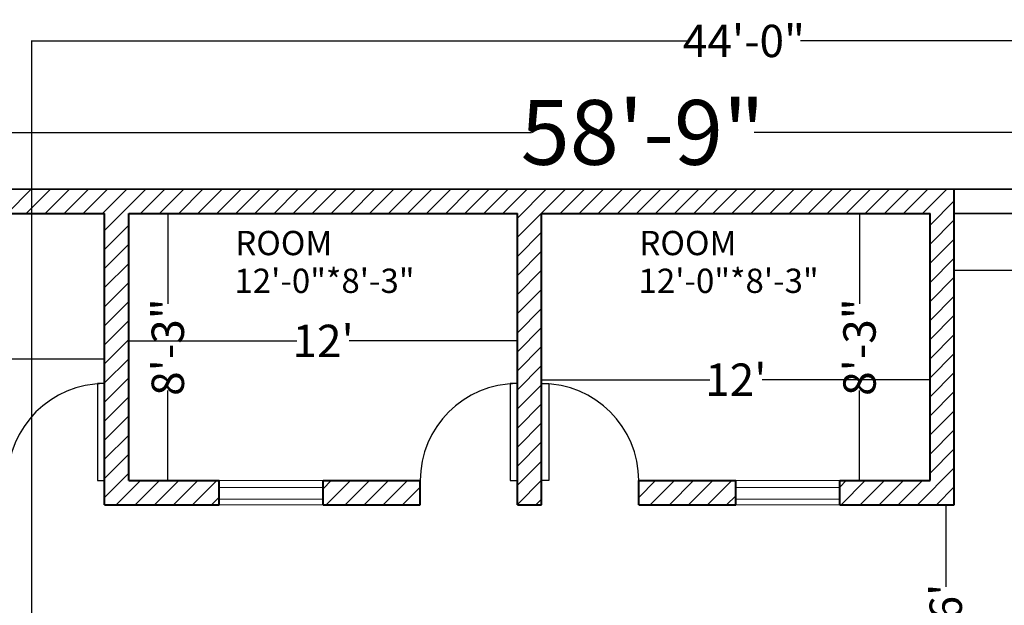
# Model space of a CAD drawing. Units: inches. Extents: x 1146 to 2917, y 889 to 2437.
# Tile 8 of 13: x 1427 to 1792, y 2217 to 2434. Entities that reach past the tile are written whole.
import ezdxf

# ---------------------------------------------------------------- set-up
doc = ezdxf.new("R2010")
doc.units = ezdxf.units.IN
doc.header["$MEASUREMENT"] = 0
for name, color, linetype, lineweight in [('A-ANNO-DIMS', 2, 'Continuous', 18), ('A-AREA-IDEN', 7, 'Continuous', 18), ('A-SITE-WALL', 7, 'Continuous', 35), ('A-WALL-PATT', 163, 'Continuous', 13), ('door', 10, 'Continuous', 25), ('wall', 7, 'Continuous', 40), ('window', 5, 'Continuous', 18)]:
    doc.layers.add(name, color=color, linetype=linetype, lineweight=lineweight)
doc.styles.get("Standard").update_dxf_attribs({"font": 'arial.ttf'})
doc.dimstyles.new('Copy of Standard', dxfattribs={"dimtxt": 24, "dimasz": 0.18, "dimexe": 0.18, "dimexo": 0.0625, "dimgap": 0.09, "dimtad": 0, "dimtoh": 1, "dimdec": 1, "dimzin": 0, "dimdsep": 46, "dimlunit": 4, "dimtxsty": 'Standard', "dimcen": 0.09, "dimadec": 0, "dimazin": 0, "dimtfac": 1, "dimtdec": 1, "dimtofl": 0, "dimtmove": 0, "dimatfit": 3, "dimfxl": 1, "dimtolj": 1, "dimtzin": 0, "dimarcsym": 0})
doc.dimstyles.get("Standard").update_dxf_attribs({"dimtxt": 12, "dimasz": 0.18, "dimexe": 0.18, "dimexo": 0.0625, "dimgap": 0.09, "dimtad": 0, "dimtoh": 1, "dimdec": 1, "dimzin": 0, "dimdsep": 46, "dimlunit": 4, "dimtxsty": 'Standard', "dimcen": 0.09, "dimadec": 0, "dimazin": 0, "dimtfac": 1, "dimtdec": 1, "dimtofl": 0, "dimtmove": 0, "dimatfit": 3, "dimfxl": 1, "dimtolj": 1, "dimtzin": 0, "dimarcsym": 0})

# ---------------------------------------------------------------- blocks, each defined once
blk = doc.blocks.new('*D2')
at = {"layer": 'A-ANNO-DIMS', "color": 0, "lineweight": -2, "transparency": 16777216}
for p, q in [((1467.2, 2362.39), (1481.72, 2362.39)), ((1481.54, 2362.21), (1481.54, 2328.94)), ((1481.54, 2263.57), (1481.54, 2296.84)), ((1467.2, 2263.39), (1481.72, 2263.39))]:
    blk.add_line(p, q, dxfattribs=at)
at = {"layer": 'A-ANNO-DIMS', "color": 0, "transparency": 16777216}
for points in [[(1481.51, 2362.21), (1481.57, 2362.21), (1481.54, 2362.39)], [(1481.51, 2263.57), (1481.57, 2263.57), (1481.54, 2263.39)]]:
    blk.add_solid(points, dxfattribs=at)
at = {"layer": 'Defpoints', "color": 0, "transparency": 16777216}
for p in [(1467.13, 2362.39), (1467.13, 2263.39), (1481.54, 2263.39)]:
    blk.add_point(p, dxfattribs=at)
at = {"layer": 'A-ANNO-DIMS', "color": 0, "transparency": 16777216, "insert": (1481.54, 2312.89), "char_height": 12, "attachment_point": 5, "rotation": 90}
blk.add_mtext('\\A1;8\'-3"', dxfattribs=at)
blk = doc.blocks.new('*D3')
at = {"layer": 'A-ANNO-DIMS', "color": 0, "lineweight": -2, "transparency": 16777216}
for p, q in [((1764.07, 2362.39), (1737.79, 2362.39)), ((1737.97, 2362.21), (1737.97, 2328.94)), ((1737.97, 2263.57), (1737.97, 2296.84)), ((1764.07, 2263.39), (1737.79, 2263.39))]:
    blk.add_line(p, q, dxfattribs=at)
at = {"layer": 'A-ANNO-DIMS', "color": 0, "transparency": 16777216}
for points in [[(1737.94, 2362.21), (1738, 2362.21), (1737.97, 2362.39)], [(1737.94, 2263.57), (1738, 2263.57), (1737.97, 2263.39)]]:
    blk.add_solid(points, dxfattribs=at)
at = {"layer": 'Defpoints', "color": 0, "transparency": 16777216}
for p in [(1764.13, 2362.39), (1737.97, 2263.39), (1764.13, 2263.39)]:
    blk.add_point(p, dxfattribs=at)
at = {"layer": 'A-ANNO-DIMS', "color": 0, "transparency": 16777216, "insert": (1737.97, 2312.89), "char_height": 12, "attachment_point": 5, "rotation": 90}
blk.add_mtext('\\A1;8\'-3"', dxfattribs=at)
blk = doc.blocks.new('*D4')
at = {"layer": 'A-ANNO-DIMS', "color": 0, "lineweight": -2, "transparency": 16777216}
for p, q in [((1620.13, 2362.33), (1620.13, 2300.64)), ((1764.13, 2362.33), (1764.13, 2300.64)), ((1620.31, 2300.82), (1682.43, 2300.82)), ((1763.95, 2300.82), (1701.84, 2300.82))]:
    blk.add_line(p, q, dxfattribs=at)
at = {"layer": 'A-ANNO-DIMS', "color": 0, "transparency": 16777216}
for points in [[(1620.31, 2300.85), (1620.31, 2300.79), (1620.13, 2300.82)], [(1763.95, 2300.85), (1763.95, 2300.79), (1764.13, 2300.82)]]:
    blk.add_solid(points, dxfattribs=at)
at = {"layer": 'Defpoints', "color": 0, "transparency": 16777216}
for p in [(1620.13, 2362.39), (1764.13, 2362.39), (1764.13, 2300.82)]:
    blk.add_point(p, dxfattribs=at)
at = {"layer": 'A-ANNO-DIMS', "color": 0, "transparency": 16777216, "insert": (1692.13, 2300.82), "char_height": 12, "attachment_point": 5}
blk.add_mtext("\\A1;12'", dxfattribs=at)
blk = doc.blocks.new('*D5')
at = {"layer": 'A-ANNO-DIMS', "color": 0, "lineweight": -2, "transparency": 16777216}
for p, q in [((1467.13, 2362.33), (1467.13, 2315.01)), ((1611.13, 2362.33), (1611.13, 2315.01)), ((1467.31, 2315.19), (1529.43, 2315.19)), ((1610.95, 2315.19), (1548.84, 2315.19))]:
    blk.add_line(p, q, dxfattribs=at)
at = {"layer": 'A-ANNO-DIMS', "color": 0, "transparency": 16777216}
for points in [[(1467.31, 2315.22), (1467.31, 2315.16), (1467.13, 2315.19)], [(1610.95, 2315.22), (1610.95, 2315.16), (1611.13, 2315.19)]]:
    blk.add_solid(points, dxfattribs=at)
at = {"layer": 'Defpoints', "color": 0, "transparency": 16777216}
for p in [(1467.13, 2362.39), (1611.13, 2362.39), (1611.13, 2315.19)]:
    blk.add_point(p, dxfattribs=at)
at = {"layer": 'A-ANNO-DIMS', "color": 0, "transparency": 16777216, "insert": (1539.13, 2315.19), "char_height": 12, "attachment_point": 5}
blk.add_mtext("\\A1;12'", dxfattribs=at)
blk = doc.blocks.new('*D6')
at = {"layer": 'A-ANNO-DIMS', "color": 0, "lineweight": -2, "transparency": 16777216}
for p, q in [((1314.13, 2362.33), (1314.13, 2308.21)), ((1458.13, 2362.33), (1458.13, 2308.21)), ((1314.31, 2308.39), (1376.43, 2308.39)), ((1457.95, 2308.39), (1395.84, 2308.39))]:
    blk.add_line(p, q, dxfattribs=at)
at = {"layer": 'A-ANNO-DIMS', "color": 0, "transparency": 16777216}
for points in [[(1314.31, 2308.42), (1314.31, 2308.36), (1314.13, 2308.39)], [(1457.95, 2308.42), (1457.95, 2308.36), (1458.13, 2308.39)]]:
    blk.add_solid(points, dxfattribs=at)
at = {"layer": 'Defpoints', "color": 0, "transparency": 16777216}
for p in [(1314.13, 2362.39), (1458.13, 2362.39), (1458.13, 2308.39)]:
    blk.add_point(p, dxfattribs=at)
at = {"layer": 'A-ANNO-DIMS', "color": 0, "transparency": 16777216, "insert": (1386.13, 2308.39), "char_height": 12, "attachment_point": 5}
blk.add_mtext("\\A1;12'", dxfattribs=at)
blk = doc.blocks.new('*U17')
for p, q in [((0, 0), (0, -6)), ((24, 0), (24, -6))]:
    blk.add_line(p, q)
blk.add_lwpolyline([(0, 0), (0, 24), (1.75, 24), (1.75, 0)], close=True)
blk.add_arc((0, 0), 24, 0, 90)
blk = doc.blocks.new('*U18')
for p, q in [((-24, 0), (-24, -6)), ((0, 0), (0, -6))]:
    blk.add_line(p, q)
blk.add_lwpolyline([(0, 0), (0, 24), (-1.75, 24), (-1.75, 0)], close=True)
blk.add_arc((0, 0), 24, 90, 180)
blk = doc.blocks.new('*D50')
at = {"layer": 'A-ANNO-DIMS', "color": 0, "lineweight": -2, "transparency": 16777216}
for p, q in [((1773.07, 2254.39), (1769.77, 2254.39)), ((1769.95, 2254.21), (1769.95, 2224.04)), ((1769.95, 2182.57), (1769.95, 2212.75)), ((1773.07, 2182.39), (1769.77, 2182.39))]:
    blk.add_line(p, q, dxfattribs=at)
at = {"layer": 'A-ANNO-DIMS', "color": 0, "transparency": 16777216}
for points in [[(1769.92, 2254.21), (1769.98, 2254.21), (1769.95, 2254.39)], [(1769.92, 2182.57), (1769.98, 2182.57), (1769.95, 2182.39)]]:
    blk.add_solid(points, dxfattribs=at)
at = {"layer": 'Defpoints', "color": 0, "transparency": 16777216}
for p in [(1773.13, 2254.39), (1769.95, 2182.39), (1773.13, 2182.39)]:
    blk.add_point(p, dxfattribs=at)
at = {"layer": 'A-ANNO-DIMS', "color": 0, "transparency": 16777216, "insert": (1769.95, 2218.39), "char_height": 12, "attachment_point": 5, "rotation": 90}
blk.add_mtext("\\A1;6'", dxfattribs=at)
blk = doc.blocks.new('*D51')
at = {"layer": 'A-ANNO-DIMS', "color": 0, "lineweight": -2, "transparency": 16777216}
for p, q in [((1773.13, 2362.33), (1773.13, 2341.24)), ((2001.13, 2362.33), (2001.13, 2341.24)), ((1773.31, 2341.42), (1877.43, 2341.42)), ((2000.95, 2341.42), (1896.84, 2341.42))]:
    blk.add_line(p, q, dxfattribs=at)
at = {"layer": 'A-ANNO-DIMS', "color": 0, "transparency": 16777216}
for points in [[(1773.31, 2341.45), (1773.31, 2341.39), (1773.13, 2341.42)], [(2000.95, 2341.45), (2000.95, 2341.39), (2001.13, 2341.42)]]:
    blk.add_solid(points, dxfattribs=at)
at = {"layer": 'Defpoints', "color": 0, "transparency": 16777216}
for p in [(1773.13, 2362.39), (2001.13, 2362.39), (2001.13, 2341.42)]:
    blk.add_point(p, dxfattribs=at)
at = {"layer": 'A-ANNO-DIMS', "color": 0, "transparency": 16777216, "insert": (1887.13, 2341.42), "char_height": 12, "attachment_point": 5}
blk.add_mtext("\\A1;19'", dxfattribs=at)
blk = doc.blocks.new('*D53')
at = {"layer": 'A-ANNO-DIMS', "color": 0, "lineweight": -2, "transparency": 16777216}
for p, q in [((1305.13, 2371.45), (1305.13, 2392.67)), ((1305.31, 2392.49), (1616.32, 2392.49)), ((2009.95, 2392.49), (1698.95, 2392.49)), ((2010.13, 2371.45), (2010.13, 2392.67))]:
    blk.add_line(p, q, dxfattribs=at)
at = {"layer": 'A-ANNO-DIMS', "color": 0, "transparency": 16777216}
for points in [[(1305.31, 2392.52), (1305.31, 2392.46), (1305.13, 2392.49)], [(2009.95, 2392.52), (2009.95, 2392.46), (2010.13, 2392.49)]]:
    blk.add_solid(points, dxfattribs=at)
at = {"layer": 'Defpoints', "color": 0, "transparency": 16777216}
for p in [(2010.13, 2392.49), (1305.13, 2371.39), (2010.13, 2371.39)]:
    blk.add_point(p, dxfattribs=at)
at = {"layer": 'A-ANNO-DIMS', "color": 0, "transparency": 16777216, "insert": (1657.63, 2392.49), "char_height": 24, "attachment_point": 5}
blk.add_mtext('\\A1;58\'-9"', dxfattribs=at)
blk = doc.blocks.new('*D168')
at = {"layer": 'A-ANNO-DIMS', "color": 0, "lineweight": -2, "transparency": 16777216}
for p, q in [((1431.13, 2029.45), (1431.13, 2426.57)), ((1431.31, 2426.39), (1674.19, 2426.39)), ((1958.95, 2426.39), (1716.08, 2426.39)), ((1959.13, 2029.45), (1959.13, 2426.57))]:
    blk.add_line(p, q, dxfattribs=at)
at = {"layer": 'A-ANNO-DIMS', "color": 0, "transparency": 16777216}
for points in [[(1431.31, 2426.42), (1431.31, 2426.36), (1431.13, 2426.39)], [(1958.95, 2426.42), (1958.95, 2426.36), (1959.13, 2426.39)]]:
    blk.add_solid(points, dxfattribs=at)
at = {"layer": 'Defpoints', "color": 0, "transparency": 16777216}
for p in [(1959.13, 2426.39), (1431.13, 2029.39), (1959.13, 2029.39)]:
    blk.add_point(p, dxfattribs=at)
at = {"layer": 'A-ANNO-DIMS', "color": 0, "transparency": 16777216, "insert": (1695.13, 2426.39), "char_height": 12, "attachment_point": 5}
blk.add_mtext('\\A1;44\'-0"', dxfattribs=at)

msp = doc.modelspace()

# ---------------------------------------------------------------- hatches: boundary and pattern name
at = {"layer": 'A-WALL-PATT'}
h = msp.add_hatch(dxfattribs=at)
h.set_pattern_fill('ANSI31', color=256, scale=40)
h.paths.add_polyline_path([(1773.13, 2371.39), (1305.13, 2371.39), (1305.13, 2362.39), (1305.13, 2254.39), (1314.13, 2254.39), (1347.63, 2254.39), (1347.63, 2263.39), (1314.13, 2263.39), (1314.13, 2362.39), (1458.13, 2362.39), (1458.13, 2254.39), (1467.13, 2254.39), (1500.63, 2254.39), (1500.63, 2263.39), (1467.13, 2263.39), (1467.13, 2362.39), (1611.13, 2362.39), (1611.13, 2254.39), (1620.13, 2254.39), (1620.13, 2362.39), (1764.13, 2362.39), (1764.13, 2263.39), (1730.63, 2263.39), (1730.63, 2254.39), (1773.13, 2254.39), (1773.13, 2362.39)])
h.paths.add_polyline_path([(1422.13, 2263.39), (1386.13, 2263.39), (1386.13, 2254.39), (1422.13, 2254.39)], flags=17)
h.paths.add_polyline_path([(1575.13, 2263.39), (1539.13, 2263.39), (1539.13, 2254.39), (1575.13, 2254.39)], flags=17)
h.paths.add_polyline_path([(1692.13, 2263.39), (1656.13, 2263.39), (1656.13, 2254.39), (1692.13, 2254.39)], flags=17)

# ---------------------------------------------------------------- linework, layer by layer
at = {"layer": 'A-SITE-WALL'}
for p, q in [((1305.13, 2371.39), (2010.13, 2371.39)), ((1773.13, 2362.39), (2001.13, 2362.39))]:
    msp.add_line(p, q, dxfattribs=at)
at = {"layer": 'wall'}
for p, q in [((1773.13, 2362.39), (1773.13, 2371.39)), ((1314.13, 2362.39), (1458.13, 2362.39)), ((1458.13, 2254.39), (1458.13, 2362.39)), ((1467.13, 2263.39), (1467.13, 2362.39)), ((1467.13, 2362.39), (1611.13, 2362.39)), ((1611.13, 2254.39), (1611.13, 2362.39)), ((1620.13, 2254.39), (1620.13, 2362.39)), ((1620.13, 2362.39), (1764.13, 2362.39)), ((1764.13, 2263.39), (1764.13, 2362.39)), ((1773.13, 2254.39), (1773.13, 2362.39)), ((1467.13, 2263.39), (1500.63, 2263.39)), ((1500.63, 2254.39), (1500.63, 2263.39)), ((1539.13, 2254.39), (1539.13, 2263.39)), ((1539.13, 2263.39), (1575.13, 2263.39)), ((1575.13, 2254.39), (1575.13, 2263.39)), ((1656.13, 2263.39), (1692.13, 2263.39)), ((1656.13, 2254.39), (1656.13, 2263.39)), ((1692.13, 2254.39), (1692.13, 2263.39)), ((1730.63, 2254.39), (1730.63, 2263.39)), ((1730.63, 2263.39), (1764.13, 2263.39)), ((1458.13, 2254.39), (1467.13, 2254.39)), ((1467.13, 2254.39), (1500.63, 2254.39)), ((1539.13, 2254.39), (1575.13, 2254.39)), ((1611.13, 2254.39), (1620.13, 2254.39)), ((1656.13, 2254.39), (1692.13, 2254.39)), ((1730.63, 2254.39), (1773.13, 2254.39))]:
    msp.add_line(p, q, dxfattribs=at)
at = {"layer": 'window'}
for points in [[(1500.63, 2263.39), (1539.13, 2263.39), (1539.13, 2254.39), (1500.63, 2254.39)], [(1692.13, 2263.39), (1730.63, 2263.39), (1730.63, 2254.39), (1692.13, 2254.39)], [(1500.63, 2260.88), (1539.13, 2260.88), (1539.13, 2256.47), (1500.63, 2256.47)], [(1692.13, 2260.88), (1730.63, 2260.88), (1730.63, 2256.47), (1692.13, 2256.47)]]:
    msp.add_lwpolyline(points, close=True, dxfattribs=at)

# ---------------------------------------------------------------- block references
at = {"layer": 'door', "xscale": 1.500000000000009, "yscale": 1.500000000000009, "zscale": 1.500000000000009}
for name, p in [('*U18', (1458.13, 2263.39)), ('*U18', (1611.13, 2263.39)), ('*U17', (1620.13, 2263.39))]:
    msp.add_blockref(name, p, dxfattribs=at)

# ---------------------------------------------------------------- texts
at = {"layer": 'A-AREA-IDEN', "char_height": 9, "attachment_point": 1}
for s, width, insert in [('ROOM', 65.2952, (1506.54, 2355.97)), ('ROOM', 65.2952, (1656.36, 2355.97)), ('12\'-0"*8\'-3"', 53.2403, (1506.22, 2341.97)), ('12\'-0"*8\'-3"', 53.2403, (1656.04, 2341.97))]:
    msp.add_mtext_dynamic_manual_height_columns(s, width=width, gutter_width=1, heights=[0], dxfattribs=dict(at, insert=insert))

# ---------------------------------------------------------------- dimensions: what is measured, and where the dimension line sits
at = {"layer": 'A-ANNO-DIMS'}
dim = msp.add_linear_dim(base=(1959.13, 2426.39), p1=(1431.13, 2029.39), p2=(1959.13, 2029.39), dimstyle='Standard', override={"dimdec": 1, "dimlfac": 1, "dimrnd": 0, "dimzin": 1, "dimdsep": 46, "dimlunit": 4, "dimfrac": 2}, dxfattribs=at)
dim.commit()
dim.dimension.update_dxf_attribs({"geometry": '*D168', "text_midpoint": (1695.13, 2426.39)})
for p1, p2, distance, dimstyle, picture, middle in [((1305.13, 2371.39), (2010.13, 2371.39), 21.1, 'Copy of Standard', '*D53', (1657.63, 2392.49)), ((1314.13, 2362.39), (1458.13, 2362.39), -54, 'Standard', '*D6', (1386.13, 2308.39)), ((1467.13, 2362.39), (1611.13, 2362.39), -47.2, 'Standard', '*D5', (1539.13, 2315.19)), ((1620.13, 2362.39), (1764.13, 2362.39), -61.57, 'Standard', '*D4', (1692.13, 2300.82)), ((1773.13, 2362.39), (2001.13, 2362.39), -20.97, 'Standard', '*D51', (1887.13, 2341.42)), ((1773.13, 2254.39), (1773.13, 2182.39), -3.19, 'Standard', '*D50', (1769.95, 2218.39))]:
    dim = msp.add_aligned_dim(p1=p1, p2=p2, distance=distance, dimstyle=dimstyle, override={"dimclrd": 0, "dimclre": 0, "dimclrt": 0}, dxfattribs=at)
    dim.commit()
    dim.dimension.update_dxf_attribs({"geometry": picture, "text_midpoint": middle})
for base, p1, p2, picture, middle in [((1481.54, 2263.39), (1467.13, 2362.39), (1467.13, 2263.39), '*D2', (1481.54, 2312.89)), ((1737.97, 2263.39), (1764.13, 2362.39), (1764.13, 2263.39), '*D3', (1737.97, 2312.89))]:
    dim = msp.add_linear_dim(base=base, p1=p1, p2=p2, angle=270, dimstyle='Standard', override={"dimclrd": 0, "dimclre": 0, "dimclrt": 0}, dxfattribs=at)
    dim.commit()
    dim.dimension.update_dxf_attribs({"geometry": picture, "text_midpoint": middle, "dimtype": 161})

doc.saveas('drawing.dxf')
